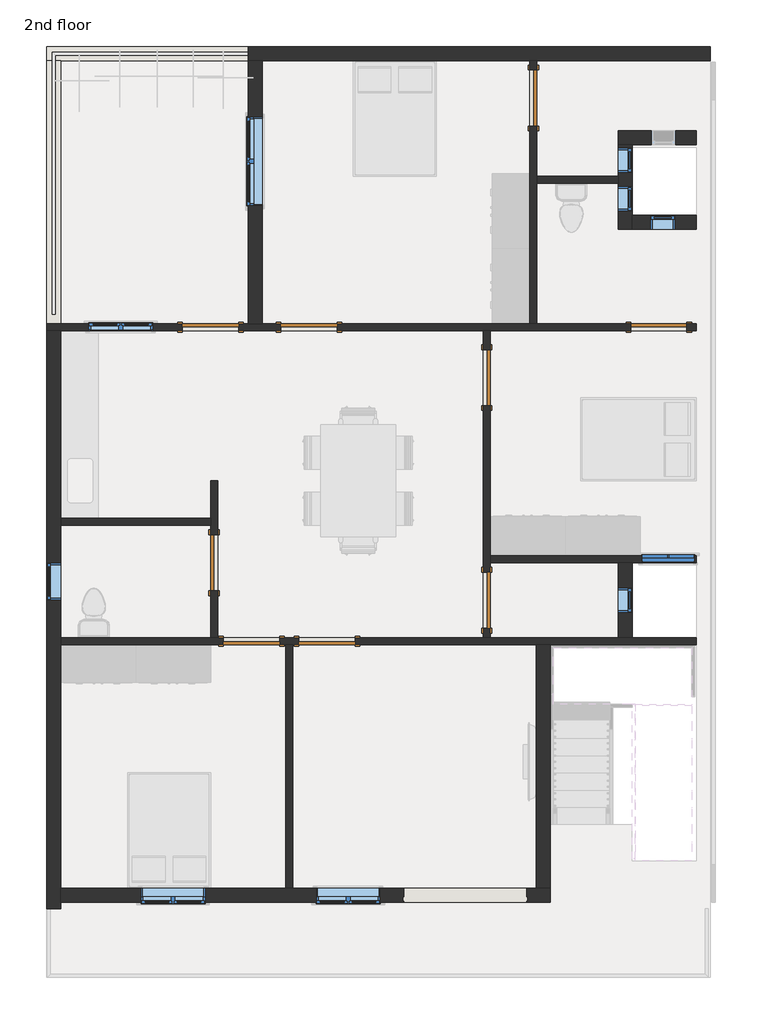
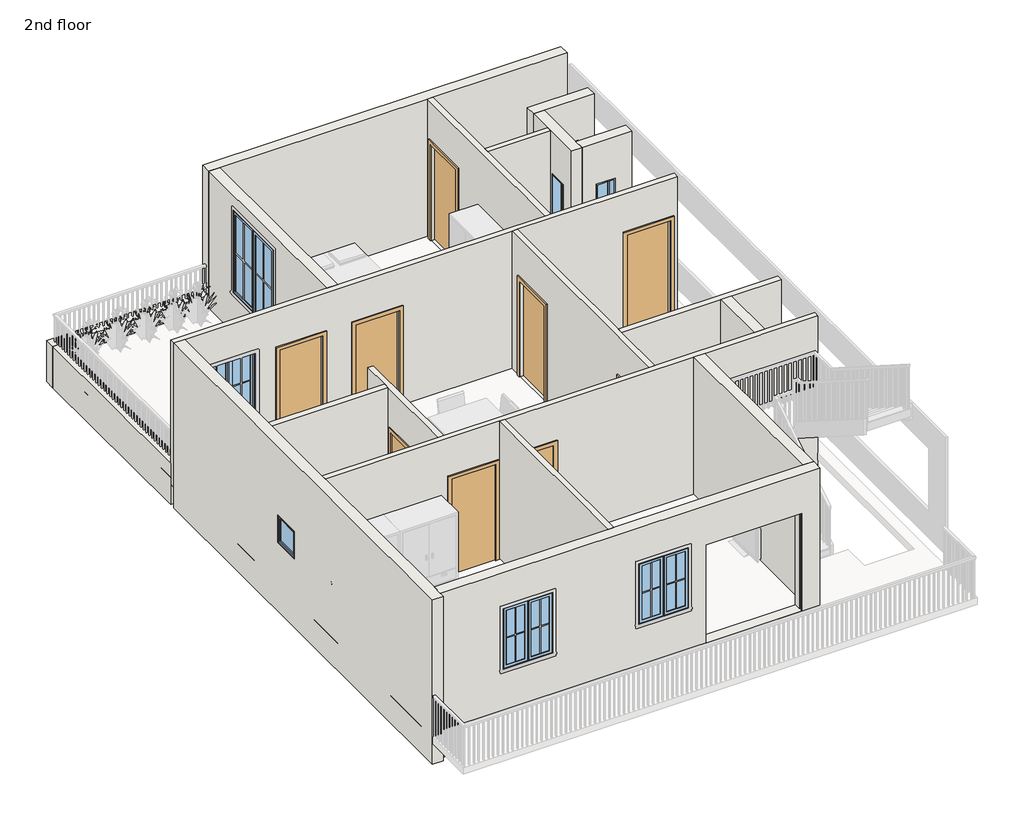
# One storey, part 1 of 5: 20 walls, 10 windows, 9 doors.
"""IFC4 building model written with IfcOpenShell, lengths in millimetres."""

from ifc_helpers import new_model, si_unit, frame, origin, place, context, project, spatial, polyline, outline, extrude, faceted_brep, transform, mapped, element, save
from components import door_305aa2a5, door_e5f9f3c4, window_aa618e30, window_cea7027f, window_80340324, window_a598f463, window_8ddb865a, window_c95ebb39, window_9ac97e1a

model = new_model("IFC4")

# Units and contexts
model_context = context("Model", 3, world=origin())
ifc_project = project(units=[si_unit("LENGTHUNIT", "METRE", prefix="MILLI")], contexts=[model_context])

# Site, building, storey
site = spatial("IfcSite", under=ifc_project)
building = spatial("IfcBuilding", under=site)
storey = spatial("IfcBuildingStorey", under=building, Name="2nd floor", Elevation=7010.4)

# Doors
placement = place(None, origin())
door_shape = door_305aa2a5(model_context)
element("IfcDoor", 1, ObjectType="Single-Flush : 36\" x 84\"", at=placement, inside=storey, context=model_context, shape_type="MappedRepresentation", body=[
    mapped(door_shape, transform((-3843.1498597, 8241.1757925, 7010.4), x_axis=(-1.0, 0.0, 0.0), y_axis=(0.0, -1.0, 0.0), z_axis=(0.0, 0.0, 1.0))),
])
element("IfcDoor", 2, ObjectType="Single-Flush : 36\" x 84\"", at=placement, inside=storey, context=model_context, shape_type="MappedRepresentation", body=[
    mapped(door_shape, transform((-953.8998597, 7422.0257925, 7010.4), x_axis=(0.0, 1.0, 0.0), y_axis=(-1.0, 0.0, 0.0), z_axis=(0.0, 0.0, 1.0))),
])
element("IfcDoor", 3, ObjectType="Single-Flush : 36\" x 84\"", at=placement, inside=storey, context=model_context, shape_type="MappedRepresentation", body=[
    mapped(door_shape, transform((-4776.5998597, 3135.7757925, 7010.4), x_axis=(1.0, 0.0, 0.0), y_axis=(0.0, 1.0, 0.0), z_axis=(0.0, 0.0, 1.0))),
])
element("IfcDoor", 4, ObjectType="Single-Flush : 36\" x 84\"", at=placement, inside=storey, context=model_context, shape_type="MappedRepresentation", body=[
    mapped(door_shape, transform((-191.8998597, 11968.6257925, 7010.4), x_axis=(0.0, 1.0, 0.0), y_axis=(-1.0, 0.0, 0.0), z_axis=(0.0, 0.0, 1.0))),
])
door_2_shape = door_e5f9f3c4(model_context)
element("IfcDoor", 5, ObjectType="Single-Flush : 36\" x 84\"", at=placement, inside=storey, context=model_context, shape_type="MappedRepresentation", body=[
    mapped(door_2_shape, transform((1846.4501403, 8241.1757925, 7010.4), x_axis=(1.0, 0.0, 0.0), y_axis=(0.0, 1.0, 0.0), z_axis=(0.0, 0.0, 1.0))),
])
element("IfcDoor", 6, ObjectType="Single-Flush : 36\" x 84\"", at=placement, inside=storey, context=model_context, shape_type="MappedRepresentation", body=[
    mapped(door_2_shape, transform((-3551.0498597, 3135.7757925, 7010.4), x_axis=(-1.0, 0.0, 0.0), y_axis=(0.0, -1.0, 0.0), z_axis=(0.0, 0.0, 1.0))),
])
element("IfcDoor", 7, ObjectType="Single-Flush : 36\" x 84\"", at=placement, inside=storey, context=model_context, shape_type="MappedRepresentation", body=[
    mapped(door_2_shape, transform((-953.8998597, 3802.5257925, 7010.4), x_axis=(0.0, -1.0, 0.0), y_axis=(1.0, 0.0, 0.0), z_axis=(0.0, 0.0, 1.0))),
])
element("IfcDoor", 8, ObjectType="Single-Flush : 36\" x 84\"", at=placement, inside=storey, context=model_context, shape_type="MappedRepresentation", body=[
    mapped(door_2_shape, transform((-5443.3498597, 8241.1757925, 7010.4), x_axis=(1.0, 0.0, 0.0), y_axis=(0.0, 1.0, 0.0), z_axis=(0.0, 0.0, 1.0))),
])
element("IfcDoor", 9, ObjectType="Single-Flush : 36\" x 84\"", at=placement, inside=storey, context=model_context, shape_type="MappedRepresentation", body=[
    mapped(door_2_shape, transform((-5386.1998597, 4412.1257925, 7010.4), x_axis=(0.0, 1.0, 0.0), y_axis=(-1.0, 0.0, 0.0), z_axis=(0.0, 0.0, 1.0))),
])

# Walls
element("IfcWall", 10, at=placement, inside=storey, context=model_context, shape_type="Brep", body=[
    faceted_brep([(-8110.3498597, 12578.2257925, 6400.8), (-7881.7498597, 12578.2257925, 6400.8), (-4833.7498597, 12578.2257925, 6400.8), (-4833.7498597, 12578.2257925, 6858.0), (-4605.1498597, 12578.2257925, 6858.0), (-4605.1498597, 12578.2257925, 7010.4), (-4719.4498597, 12578.2257925, 7010.4), (-4719.4498597, 12578.2257925, 7315.2), (-4833.7498597, 12578.2257925, 7315.2), (-7881.7498597, 12578.2257925, 7315.2), (-8110.3498597, 12578.2257925, 7315.2), (-8110.3498597, 12806.8257925, 6400.8), (-8110.3498597, 12806.8257925, 7315.2), (-4833.7498597, 12806.8257925, 7315.2), (-4719.4498597, 12806.8257925, 7315.2), (-4719.4498597, 12806.8257925, 7010.4), (-4605.1498597, 12806.8257925, 7010.4), (-4605.1498597, 12806.8257925, 6858.0), (-4833.7498597, 12806.8257925, 6858.0), (-4833.7498597, 12806.8257925, 6400.8)], [[[0, 1, 2, 3, 4, 5, 6, 7, 8, 9, 10]], [[11, 12, 13, 14, 15, 16, 17, 18, 19]], [[2, 1, 0, 11, 19]], [[10, 9, 8, 7, 14, 13, 12]], [[0, 10, 12, 11]], [[3, 2, 19, 18]], [[17, 4, 3, 18]], [[7, 6, 15, 14]], [[15, 6, 5, 16]], [[5, 4, 17, 16]]]),
])
element("IfcWall", 11, at=placement, inside=storey, context=model_context, shape_type="Brep", body=[
    faceted_brep([(-4833.7498597, 12578.2257925, 10058.4), (-4833.7498597, 12578.2257925, 7315.2), (-4833.7498597, 12578.2257925, 6858.0), (-4833.7498597, 12578.2257925, 6400.8), (-4833.7498597, 8298.3257925, 6400.8), (-4833.7498597, 8298.3257925, 10058.4), (-4833.7498597, 11663.8257925, 9753.6), (-4833.7498597, 10216.0257925, 9753.6), (-4833.7498597, 10216.0257925, 7924.8), (-4833.7498597, 11663.8257925, 7924.8), (-4605.1498597, 12578.2257925, 6400.8), (-4605.1498597, 12578.2257925, 6858.0), (-4605.1498597, 12578.2257925, 7010.4), (-4605.1498597, 12578.2257925, 10058.4), (-4605.1498597, 8298.3257925, 10058.4), (-4605.1498597, 8298.3257925, 6400.8), (-4605.1498597, 11663.8257925, 9753.6), (-4605.1498597, 11663.8257925, 7924.8), (-4605.1498597, 10216.0257925, 7924.8), (-4605.1498597, 10216.0257925, 9753.6)], [[[0, 1, 2, 3, 4, 5], [6, 7, 8, 9]], [[10, 11, 12, 13, 14, 15], [16, 17, 18, 19]], [[4, 3, 10, 15]], [[17, 16, 6, 9]], [[18, 17, 9, 8]], [[19, 18, 8, 7]], [[16, 19, 7, 6]], [[4, 15, 14, 5]], [[0, 13, 12, 11, 10, 3, 2, 1]], [[0, 5, 14, 13]]]),
])
element("IfcWall", 12, at=placement, inside=storey, context=model_context, shape_type="Brep", body=[
    faceted_brep([(2456.0501403, 8298.3257925, 6400.8), (-134.7498597, 8298.3257925, 6400.8), (-249.0498597, 8298.3257925, 6400.8), (-4605.1498597, 8298.3257925, 6400.8), (-4833.7498597, 8298.3257925, 6400.8), (-7881.7498597, 8298.3257925, 6400.8), (-7881.7498597, 8298.3257925, 6858.0), (-8110.3498597, 8298.3257925, 6858.0), (-8110.3498597, 8298.3257925, 7315.2), (-8110.3498597, 8298.3257925, 10058.4), (-4833.7498597, 8298.3257925, 10058.4), (-4605.1498597, 8298.3257925, 10058.4), (-249.0498597, 8298.3257925, 10058.4), (-134.7498597, 8298.3257925, 10058.4), (2456.0501403, 8298.3257925, 10058.4), (1389.2501403, 8298.3257925, 7010.4), (2303.6501403, 8298.3257925, 7010.4), (2303.6501403, 8298.3257925, 9144.0), (1389.2501403, 8298.3257925, 9144.0), (-3385.9498597, 8298.3257925, 7010.4), (-3385.9498597, 8298.3257925, 9144.0), (-4300.3498597, 8298.3257925, 9144.0), (-4300.3498597, 8298.3257925, 7010.4), (-5900.5498597, 8298.3257925, 7010.4), (-4986.1498597, 8298.3257925, 7010.4), (-4986.1498597, 8298.3257925, 9144.0), (-5900.5498597, 8298.3257925, 9144.0), (-6383.1498597, 8298.3257925, 9271.0), (-7424.5498597, 8298.3257925, 9271.0), (-7424.5498597, 8298.3257925, 7924.8), (-6383.1498597, 8298.3257925, 7924.8), (2456.0501403, 8184.0257925, 6400.8), (2456.0501403, 8184.0257925, 10058.4), (-896.7498597, 8184.0257925, 10058.4), (-1011.0498597, 8184.0257925, 10058.4), (-7881.7498597, 8184.0257925, 10058.4), (-8110.3498597, 8184.0257925, 10058.4), (-8110.3498597, 8184.0257925, 6858.0), (-7881.7498597, 8184.0257925, 6858.0), (-7881.7498597, 8184.0257925, 6400.8), (-1011.0498597, 8184.0257925, 6400.8), (-896.7498597, 8184.0257925, 6400.8), (1389.2501403, 8184.0257925, 7010.4), (1389.2501403, 8184.0257925, 9144.0), (2303.6501403, 8184.0257925, 9144.0), (2303.6501403, 8184.0257925, 7010.4), (-3385.9498597, 8184.0257925, 7010.4), (-4300.3498597, 8184.0257925, 7010.4), (-4300.3498597, 8184.0257925, 9144.0), (-3385.9498597, 8184.0257925, 9144.0), (-5900.5498597, 8184.0257925, 7010.4), (-5900.5498597, 8184.0257925, 9144.0), (-4986.1498597, 8184.0257925, 9144.0), (-4986.1498597, 8184.0257925, 7010.4), (-6383.1498597, 8184.0257925, 9271.0), (-6383.1498597, 8184.0257925, 7924.8), (-7424.5498597, 8184.0257925, 7924.8), (-7424.5498597, 8184.0257925, 9271.0)], [[[0, 1, 2, 3, 4, 5, 6, 7, 8, 9, 10, 11, 12, 13, 14], [15, 16, 17, 18], [19, 20, 21, 22], [23, 24, 25, 26], [27, 28, 29, 30]], [[31, 32, 33, 34, 35, 36, 37, 38, 39, 40, 41], [42, 43, 44, 45], [46, 47, 48, 49], [50, 51, 52, 53], [54, 55, 56, 57]], [[5, 4, 3, 2, 1, 0, 31, 41, 40, 39]], [[16, 15, 42, 45]], [[17, 16, 45, 44]], [[18, 17, 44, 43]], [[15, 18, 43, 42]], [[47, 46, 19, 22]], [[48, 47, 22, 21]], [[49, 48, 21, 20]], [[46, 49, 20, 19]], [[24, 23, 50, 53]], [[25, 24, 53, 52]], [[26, 25, 52, 51]], [[23, 26, 51, 50]], [[55, 54, 27, 30]], [[56, 55, 30, 29]], [[57, 56, 29, 28]], [[54, 57, 28, 27]], [[37, 7, 6, 38]], [[6, 5, 39, 38]], [[7, 37, 36, 9, 8]], [[0, 14, 32, 31]], [[14, 13, 12, 11, 10, 9, 36, 35, 34, 33, 32]]]),
])
element("IfcWall", 13, at=placement, inside=storey, context=model_context, shape_type="Brep", body=[
    faceted_brep([(2456.0501403, 11435.2257925, 6400.8), (1414.6501403, 11435.2257925, 6400.8), (1414.6501403, 11435.2257925, 6858.0), (1186.0501403, 11435.2257925, 6858.0), (1186.0501403, 11435.2257925, 10058.4), (2456.0501403, 11435.2257925, 10058.4), (1719.4501403, 11435.2257925, 9144.0), (1719.4501403, 11435.2257925, 7924.8), (2125.8501403, 11435.2257925, 7924.8), (2125.8501403, 11435.2257925, 9144.0), (2456.0501403, 11206.6257925, 6400.8), (2456.0501403, 11206.6257925, 10058.4), (1414.6501403, 11206.6257925, 10058.4), (1186.0501403, 11206.6257925, 10058.4), (1186.0501403, 11206.6257925, 6858.0), (1414.6501403, 11206.6257925, 6858.0), (1414.6501403, 11206.6257925, 6400.8), (1719.4501403, 11206.6257925, 9144.0), (2125.8501403, 11206.6257925, 9144.0), (2125.8501403, 11206.6257925, 7924.8), (1719.4501403, 11206.6257925, 7924.8)], [[[0, 1, 2, 3, 4, 5], [6, 7, 8, 9]], [[10, 11, 12, 13, 14, 15, 16], [17, 18, 19, 20]], [[1, 0, 10, 16]], [[7, 6, 17, 20]], [[8, 7, 20, 19]], [[9, 8, 19, 18]], [[6, 9, 18, 17]], [[14, 3, 2, 15]], [[2, 1, 16, 15]], [[4, 3, 14, 13]], [[0, 5, 11, 10]], [[5, 4, 13, 12, 11]]]),
])
element("IfcWall", 14, at=placement, inside=storey, context=model_context, shape_type="Brep", body=[
    faceted_brep([(1186.0501403, 11206.6257925, 6400.8), (1186.0501403, 10698.6257925, 6400.8), (1186.0501403, 10584.3257925, 6400.8), (1186.0501403, 10063.6257925, 6400.8), (1186.0501403, 10063.6257925, 6858.0), (1186.0501403, 9835.0257925, 6858.0), (1186.0501403, 9835.0257925, 10058.4), (1186.0501403, 10584.3257925, 10058.4), (1186.0501403, 10698.6257925, 10058.4), (1186.0501403, 11206.6257925, 10058.4), (1186.0501403, 11206.6257925, 6858.0), (1186.0501403, 10127.1257925, 9144.0), (1186.0501403, 10127.1257925, 7924.8), (1186.0501403, 10533.5257925, 7924.8), (1186.0501403, 10533.5257925, 9144.0), (1186.0501403, 10755.7299127, 9144.0), (1186.0501403, 10755.7299127, 7924.8), (1186.0501403, 11162.1299127, 7924.8), (1186.0501403, 11162.1299127, 9144.0), (1414.6501403, 10063.6257925, 6400.8), (1414.6501403, 11206.6257925, 6400.8), (1414.6501403, 11206.6257925, 10058.4), (1414.6501403, 10063.6257925, 10058.4), (1414.6501403, 9835.0257925, 10058.4), (1414.6501403, 9835.0257925, 6858.0), (1414.6501403, 10063.6257925, 6858.0), (1414.6501403, 10127.1257925, 7924.8), (1414.6501403, 10127.1257925, 9144.0), (1414.6501403, 10533.5257925, 9144.0), (1414.6501403, 10533.5257925, 7924.8), (1414.6501403, 10755.7299127, 7924.8), (1414.6501403, 10755.7299127, 9144.0), (1414.6501403, 11162.1299127, 9144.0), (1414.6501403, 11162.1299127, 7924.8)], [[[0, 1, 2, 3, 4, 5, 6, 7, 8, 9, 10], [11, 12, 13, 14], [15, 16, 17, 18]], [[19, 20, 21, 22, 23, 24, 25], [26, 27, 28, 29], [30, 31, 32, 33]], [[3, 2, 1, 0, 20, 19]], [[12, 11, 27, 26]], [[13, 12, 26, 29]], [[14, 13, 29, 28]], [[11, 14, 28, 27]], [[15, 31, 30, 16]], [[16, 30, 33, 17]], [[31, 15, 18, 32]], [[32, 18, 17, 33]], [[20, 0, 10, 9, 21]], [[5, 4, 25, 24]], [[4, 3, 19, 25]], [[6, 5, 24, 23]], [[21, 9, 8, 7, 6, 23, 22]]]),
])
element("IfcWall", 15, at=placement, inside=storey, context=model_context, shape_type="Brep", body=[
    faceted_brep([(1414.6501403, 9835.0257925, 10058.4), (1414.6501403, 9835.0257925, 6858.0), (1414.6501403, 9835.0257925, 6400.8), (2456.0501403, 9835.0257925, 6400.8), (2456.0501403, 9835.0257925, 10058.4), (2113.1501403, 9835.0257925, 9144.0), (2113.1501403, 9835.0257925, 7924.8), (1706.7501403, 9835.0257925, 7924.8), (1706.7501403, 9835.0257925, 9144.0), (1414.6501403, 10063.6257925, 6400.8), (1414.6501403, 10063.6257925, 10058.4), (2456.0501403, 10063.6257925, 10058.4), (2456.0501403, 10063.6257925, 6400.8), (2113.1501403, 10063.6257925, 9144.0), (1706.7501403, 10063.6257925, 9144.0), (1706.7501403, 10063.6257925, 7924.8), (2113.1501403, 10063.6257925, 7924.8)], [[[0, 1, 2, 3, 4], [5, 6, 7, 8]], [[9, 10, 11, 12], [13, 14, 15, 16]], [[3, 2, 9, 12]], [[6, 5, 13, 16]], [[7, 6, 16, 15]], [[8, 7, 15, 14]], [[5, 8, 14, 13]], [[0, 10, 9, 2, 1]], [[4, 3, 12, 11]], [[0, 4, 11, 10]]]),
])
element("IfcWall", 16, at=placement, inside=storey, context=model_context, shape_type="Brep", body=[
    faceted_brep([(-7881.7498597, 3078.6257925, 10058.4), (-7881.7498597, 3078.6257925, 6400.8), (-4224.1498597, 3078.6257925, 6400.8), (-4109.8498597, 3078.6257925, 6400.8), (-147.4498597, 3078.6257925, 6400.8), (81.1501403, 3078.6257925, 6400.8), (2456.0501403, 3078.6257925, 6400.8), (2456.0501403, 3078.6257925, 10058.4), (2430.6501403, 3078.6257925, 10058.4), (81.1501403, 3078.6257925, 10058.4), (-147.4498597, 3078.6257925, 10058.4), (-4109.8498597, 3078.6257925, 10058.4), (-4224.1498597, 3078.6257925, 10058.4), (-5233.7998597, 3078.6257925, 7010.4), (-5233.7998597, 3078.6257925, 9144.0), (-4319.3998597, 3078.6257925, 9144.0), (-4319.3998597, 3078.6257925, 7010.4), (-3093.8498597, 3078.6257925, 7010.4), (-4008.2498597, 3078.6257925, 7010.4), (-4008.2498597, 3078.6257925, 9144.0), (-3093.8498597, 3078.6257925, 9144.0), (-7881.7498597, 3192.9257925, 6400.8), (-7881.7498597, 3192.9257925, 10058.4), (-5443.3498597, 3192.9257925, 10058.4), (-5329.0498597, 3192.9257925, 10058.4), (-1011.0498597, 3192.9257925, 10058.4), (-896.7498597, 3192.9257925, 10058.4), (1186.0501403, 3192.9257925, 10058.4), (1414.6501403, 3192.9257925, 10058.4), (2456.0501403, 3192.9257925, 10058.4), (2456.0501403, 3192.9257925, 6400.8), (1414.6501403, 3192.9257925, 6400.8), (1186.0501403, 3192.9257925, 6400.8), (-896.7498597, 3192.9257925, 6400.8), (-1011.0498597, 3192.9257925, 6400.8), (-5329.0498597, 3192.9257925, 6400.8), (-5443.3498597, 3192.9257925, 6400.8), (-5233.7998597, 3192.9257925, 7010.4), (-4319.3998597, 3192.9257925, 7010.4), (-4319.3998597, 3192.9257925, 9144.0), (-5233.7998597, 3192.9257925, 9144.0), (-3093.8498597, 3192.9257925, 7010.4), (-3093.8498597, 3192.9257925, 9144.0), (-4008.2498597, 3192.9257925, 9144.0), (-4008.2498597, 3192.9257925, 7010.4)], [[[0, 1, 2, 3, 4, 5, 6, 7, 8, 9, 10, 11, 12], [13, 14, 15, 16], [17, 18, 19, 20]], [[21, 22, 23, 24, 25, 26, 27, 28, 29, 30, 31, 32, 33, 34, 35, 36], [37, 38, 39, 40], [41, 42, 43, 44]], [[6, 5, 4, 3, 2, 1, 21, 36, 35, 34, 33, 32, 31, 30]], [[38, 37, 13, 16]], [[39, 38, 16, 15]], [[40, 39, 15, 14]], [[37, 40, 14, 13]], [[18, 17, 41, 44]], [[19, 18, 44, 43]], [[20, 19, 43, 42]], [[17, 20, 42, 41]], [[0, 22, 21, 1]], [[7, 6, 30, 29]], [[0, 12, 11, 10, 9, 8, 7, 29, 28, 27, 26, 25, 24, 23, 22]]]),
])
element("IfcWall", 17, at=placement, inside=storey, context=model_context, shape_type="Brep", body=[
    faceted_brep([(-7881.7498597, -1112.3742075, 6400.8), (-147.4498597, -1112.3742075, 6400.8), (-147.4498597, -1112.3742075, 6858.0), (81.1501403, -1112.3742075, 6858.0), (81.1501403, -1112.3742075, 10058.4), (-7881.7498597, -1112.3742075, 10058.4), (-2299.8498597, -1112.3742075, 9179.9), (-299.8498597, -1112.3742075, 9179.9), (-299.8498597, -1112.3742075, 7010.4), (-2299.8498597, -1112.3742075, 7010.4), (-6573.6498597, -1112.3742075, 7924.8), (-6573.6498597, -1112.3742075, 9271.0), (-5532.2498597, -1112.3742075, 9271.0), (-5532.2498597, -1112.3742075, 7924.8), (-3725.5498597, -1112.3742075, 7924.8), (-3725.5498597, -1112.3742075, 9271.0), (-2684.1498597, -1112.3742075, 9271.0), (-2684.1498597, -1112.3742075, 7924.8), (-147.4498597, -883.7742075, 6400.8), (-4109.8498597, -883.7742075, 6400.8), (-4224.1498597, -883.7742075, 6400.8), (-7881.7498597, -883.7742075, 6400.8), (-7881.7498597, -883.7742075, 10058.4), (-4224.1498597, -883.7742075, 10058.4), (-4109.8498597, -883.7742075, 10058.4), (-147.4498597, -883.7742075, 10058.4), (81.1501403, -883.7742075, 10058.4), (81.1501403, -883.7742075, 6858.0), (-147.4498597, -883.7742075, 6858.0), (-299.8498597, -883.7742075, 9179.9), (-2299.8498597, -883.7742075, 9179.9), (-2299.8498597, -883.7742075, 7010.4), (-299.8498597, -883.7742075, 7010.4), (-6573.6498597, -883.7742075, 9271.0), (-6573.6498597, -883.7742075, 7924.8), (-5532.2498597, -883.7742075, 7924.8), (-5532.2498597, -883.7742075, 9271.0), (-3725.5498597, -883.7742075, 9271.0), (-3725.5498597, -883.7742075, 7924.8), (-2684.1498597, -883.7742075, 7924.8), (-2684.1498597, -883.7742075, 9271.0), (-2299.8498597, -1092.3742075, 9179.9), (-299.8498597, -1092.3742075, 9179.9), (-299.8498597, -1022.3742075, 9179.9), (-2299.8498597, -1022.3742075, 9179.9), (-2299.8498597, -1022.3742075, 7010.4), (-2314.8498597, -1022.3742075, 7010.4), (-2314.8498597, -1092.3742075, 7010.4), (-2299.8498597, -1092.3742075, 7010.4), (-299.8498597, -1092.3742075, 7010.4), (-284.8498597, -1092.3742075, 7010.4), (-284.8498597, -1022.3742075, 7010.4), (-299.8498597, -1022.3742075, 7010.4), (-284.8498597, -1022.3742075, 9194.9), (-2314.8498597, -1022.3742075, 9194.9), (-2314.8498597, -1092.3742075, 9194.9), (-284.8498597, -1092.3742075, 9194.9)], [[[0, 1, 2, 3, 4, 5], [6, 7, 8, 9], [10, 11, 12, 13], [14, 15, 16, 17]], [[18, 19, 20, 21, 22, 23, 24, 25, 26, 27, 28], [29, 30, 31, 32], [33, 34, 35, 36], [37, 38, 39, 40]], [[1, 0, 21, 20, 19, 18]], [[41, 42, 7, 6]], [[43, 44, 30, 29]], [[45, 46, 47, 48, 9, 8, 49, 50, 51, 52, 32, 31]], [[52, 43, 29, 32]], [[44, 45, 31, 30]], [[44, 43, 52, 51, 53, 54, 46, 45]], [[47, 46, 54, 55]], [[42, 41, 48, 47, 55, 56, 50, 49]], [[48, 41, 6, 9]], [[42, 49, 8, 7]], [[51, 50, 56, 53]], [[54, 53, 56, 55]], [[34, 33, 11, 10]], [[35, 34, 10, 13]], [[36, 35, 13, 12]], [[33, 36, 12, 11]], [[38, 37, 15, 14]], [[39, 38, 14, 17]], [[40, 39, 17, 16]], [[37, 40, 16, 15]], [[21, 0, 5, 22]], [[3, 2, 28, 27]], [[2, 1, 18, 28]], [[4, 3, 27, 26]], [[5, 4, 26, 25, 24, 23, 22]]]),
])
element("IfcWall", 18, at=placement, inside=storey, context=model_context, shape_type="SweptSolid", body=[
    extrude(outline(polyline([(-4109.8498597, 3078.6257925), (-4109.8498597, -883.7742075), (-4224.1498597, -883.7742075), (-4224.1498597, 3078.6257925), (-4109.8498597, 3078.6257925)])), frame((0.0, 0.0, 6400.8), z_axis=(0.0, 0.0, 1.0), x_axis=(1.0, 0.0, 0.0)), (0.0, 0.0, 1.0), 3657.6),
])
element("IfcWall", 19, at=placement, inside=storey, context=model_context, shape_type="Brep", body=[
    faceted_brep([(81.1501403, -883.7742075, 10058.4), (81.1501403, -883.7742075, 6858.0), (81.1501403, -883.7742075, 6400.8), (81.1501403, 3078.6257925, 6400.8), (81.1501403, 3078.6257925, 10058.4), (81.1501403, 157.6257925, 10058.4), (-147.4498597, -883.7742075, 6400.8), (-147.4498597, -883.7742075, 10058.4), (-147.4498597, 3078.6257925, 10058.4), (-147.4498597, 3078.6257925, 6400.8)], [[[0, 1, 2, 3, 4, 5]], [[6, 7, 8, 9]], [[3, 2, 6, 9]], [[3, 9, 8, 4]], [[0, 7, 6, 2, 1]], [[0, 5, 4, 8, 7]]]),
])
element("IfcWall", 20, at=placement, inside=storey, context=model_context, shape_type="SweptSolid", body=[
    extrude(outline(polyline([(3192.9257925, 6400.8), (3192.9257925, 10058.4), (4412.1257925, 10058.4), (4412.1257925, 6400.8), (3192.9257925, 6400.8)]), holes=[polyline([(3599.3257925, 8534.4), (3599.3257925, 7924.8), (4005.7257925, 7924.8), (4005.7257925, 8534.4), (3599.3257925, 8534.4)])]), frame((1186.0501403, 0.0, 0.0), z_axis=(1.0, 0.0, 0.0), x_axis=(0.0, 1.0, 0.0)), (0.0, 0.0, 1.0), 228.6),
])
element("IfcWall", 21, at=placement, inside=storey, context=model_context, shape_type="Brep", body=[
    faceted_brep([(-896.7498597, 3192.9257925, 10058.4), (-896.7498597, 3192.9257925, 6400.8), (-896.7498597, 4412.1257925, 6400.8), (-896.7498597, 4526.4257925, 6400.8), (-896.7498597, 8184.0257925, 6400.8), (-896.7498597, 8184.0257925, 10058.4), (-896.7498597, 4526.4257925, 10058.4), (-896.7498597, 4412.1257925, 10058.4), (-896.7498597, 6964.8257925, 7010.4), (-896.7498597, 6964.8257925, 9144.0), (-896.7498597, 7879.2257925, 9144.0), (-896.7498597, 7879.2257925, 7010.4), (-896.7498597, 4259.7257925, 7010.4), (-896.7498597, 3345.3257925, 7010.4), (-896.7498597, 3345.3257925, 9144.0), (-896.7498597, 4259.7257925, 9144.0), (-1011.0498597, 3192.9257925, 6400.8), (-1011.0498597, 3192.9257925, 10058.4), (-1011.0498597, 8184.0257925, 10058.4), (-1011.0498597, 8184.0257925, 6400.8), (-1011.0498597, 6964.8257925, 7010.4), (-1011.0498597, 7879.2257925, 7010.4), (-1011.0498597, 7879.2257925, 9144.0), (-1011.0498597, 6964.8257925, 9144.0), (-1011.0498597, 4259.7257925, 7010.4), (-1011.0498597, 4259.7257925, 9144.0), (-1011.0498597, 3345.3257925, 9144.0), (-1011.0498597, 3345.3257925, 7010.4)], [[[0, 1, 2, 3, 4, 5, 6, 7], [8, 9, 10, 11], [12, 13, 14, 15]], [[16, 17, 18, 19], [20, 21, 22, 23], [24, 25, 26, 27]], [[4, 3, 2, 1, 16, 19]], [[21, 20, 8, 11]], [[22, 21, 11, 10]], [[23, 22, 10, 9]], [[20, 23, 9, 8]], [[13, 12, 24, 27]], [[14, 13, 27, 26]], [[15, 14, 26, 25]], [[12, 15, 25, 24]], [[4, 19, 18, 5]], [[0, 17, 16, 1]], [[0, 7, 6, 5, 18, 17]]]),
])
element("IfcWall", 22, at=placement, inside=storey, context=model_context, shape_type="Brep", body=[
    faceted_brep([(-7881.7498597, -1213.9742075, 6400.8), (-7881.7498597, -1112.3742075, 6400.8), (-7881.7498597, -883.7742075, 6400.8), (-7881.7498597, 3078.6257925, 6400.8), (-7881.7498597, 3192.9257925, 6400.8), (-7881.7498597, 5021.7257925, 6400.8), (-7881.7498597, 5136.0257925, 6400.8), (-7881.7498597, 8184.0257925, 6400.8), (-7881.7498597, 8184.0257925, 10058.4), (-7881.7498597, 5136.0257925, 10058.4), (-7881.7498597, 5021.7257925, 10058.4), (-7881.7498597, 3192.9257925, 10058.4), (-7881.7498597, 3078.6257925, 10058.4), (-7881.7498597, -883.7742075, 10058.4), (-7881.7498597, -1112.3742075, 10058.4), (-7881.7498597, -1213.9742075, 10058.4), (-7881.7498597, 4412.1257925, 8534.4), (-7881.7498597, 4412.1257925, 7924.8), (-7881.7498597, 3802.5257925, 7924.8), (-7881.7498597, 3802.5257925, 8534.4), (-8110.3498597, -1213.9742075, 6400.8), (-8110.3498597, -1213.9742075, 10058.4), (-8110.3498597, 8184.0257925, 10058.4), (-8110.3498597, 8184.0257925, 6858.0), (-8110.3498597, 8184.0257925, 6400.8), (-8110.3498597, 4412.1257925, 8534.4), (-8110.3498597, 3802.5257925, 8534.4), (-8110.3498597, 3802.5257925, 7924.8), (-8110.3498597, 4412.1257925, 7924.8)], [[[0, 1, 2, 3, 4, 5, 6, 7, 8, 9, 10, 11, 12, 13, 14, 15], [16, 17, 18, 19]], [[20, 21, 22, 23, 24], [25, 26, 27, 28]], [[7, 6, 5, 4, 3, 2, 1, 0, 20, 24]], [[0, 15, 21, 20]], [[16, 19, 26, 25]], [[19, 18, 27, 26]], [[18, 17, 28, 27]], [[17, 16, 25, 28]], [[7, 24, 23, 22, 8]], [[15, 14, 13, 12, 11, 10, 9, 8, 22, 21]]]),
])
element("IfcWall", 23, at=placement, inside=storey, context=model_context, shape_type="Brep", body=[
    faceted_brep([(-7881.7498597, 8298.3257925, 7315.2), (-7881.7498597, 8298.3257925, 6400.8), (-7881.7498597, 12578.2257925, 6400.8), (-7881.7498597, 12578.2257925, 7315.2), (-8110.3498597, 8298.3257925, 6400.8), (-8110.3498597, 8298.3257925, 6858.0), (-8110.3498597, 8298.3257925, 7315.2), (-8110.3498597, 12578.2257925, 7315.2), (-8110.3498597, 12578.2257925, 6400.8)], [[[0, 1, 2, 3]], [[4, 5, 6, 7, 8]], [[2, 1, 4, 8]], [[0, 3, 7, 6]], [[3, 2, 8, 7]], [[0, 6, 5, 4, 1]]]),
])
element("IfcWall", 24, at=placement, inside=storey, context=model_context, shape_type="Brep", body=[
    faceted_brep([(-4719.4498597, 12578.2257925, 7010.4), (-4605.1498597, 12578.2257925, 7010.4), (2684.6501403, 12578.2257925, 7010.4), (2684.6501403, 12578.2257925, 10058.4), (-134.7498597, 12578.2257925, 10058.4), (-249.0498597, 12578.2257925, 10058.4), (-4605.1498597, 12578.2257925, 10058.4), (-4833.7498597, 12578.2257925, 10058.4), (-4833.7498597, 12578.2257925, 7315.2), (-4719.4498597, 12578.2257925, 7315.2), (-4719.4498597, 12806.8257925, 7010.4), (-4719.4498597, 12806.8257925, 7315.2), (-4833.7498597, 12806.8257925, 7315.2), (-4833.7498597, 12806.8257925, 10058.4), (2684.6501403, 12806.8257925, 10058.4), (2684.6501403, 12806.8257925, 7010.4), (-4605.1498597, 12806.8257925, 7010.4)], [[[0, 1, 2, 3, 4, 5, 6, 7, 8, 9]], [[10, 11, 12, 13, 14, 15, 16]], [[2, 1, 0, 10, 16, 15]], [[0, 9, 11, 10]], [[8, 12, 11, 9]], [[3, 2, 15, 14]], [[8, 7, 13, 12]], [[7, 6, 5, 4, 3, 14, 13]]]),
])
element("IfcWall", 25, at=placement, inside=storey, context=model_context, shape_type="Brep", body=[
    faceted_brep([(-249.0498597, 12578.2257925, 10058.4), (-249.0498597, 12578.2257925, 6400.8), (-249.0498597, 8298.3257925, 6400.8), (-249.0498597, 8298.3257925, 10058.4), (-249.0498597, 11511.4257925, 7010.4), (-249.0498597, 12425.8257925, 7010.4), (-249.0498597, 12425.8257925, 9144.0), (-249.0498597, 11511.4257925, 9144.0), (-134.7498597, 12578.2257925, 6400.8), (-134.7498597, 12578.2257925, 10058.4), (-134.7498597, 10698.6257925, 10058.4), (-134.7498597, 10584.3257925, 10058.4), (-134.7498597, 8298.3257925, 10058.4), (-134.7498597, 8298.3257925, 6400.8), (-134.7498597, 10584.3257925, 6400.8), (-134.7498597, 10698.6257925, 6400.8), (-134.7498597, 11511.4257925, 7010.4), (-134.7498597, 11511.4257925, 9144.0), (-134.7498597, 12425.8257925, 9144.0), (-134.7498597, 12425.8257925, 7010.4)], [[[0, 1, 2, 3], [4, 5, 6, 7]], [[8, 9, 10, 11, 12, 13, 14, 15], [16, 17, 18, 19]], [[2, 1, 8, 15, 14, 13]], [[5, 4, 16, 19]], [[6, 5, 19, 18]], [[7, 6, 18, 17]], [[4, 7, 17, 16]], [[0, 3, 12, 11, 10, 9]], [[2, 13, 12, 3]], [[0, 9, 8, 1]]]),
])
element("IfcWall", 26, at=placement, inside=storey, context=model_context, shape_type="SweptSolid", body=[
    extrude(outline(polyline([(-134.7498597, 10698.6257925), (1186.0501403, 10698.6257925), (1186.0501403, 10584.3257925), (-134.7498597, 10584.3257925), (-134.7498597, 10698.6257925)])), frame((0.0, 0.0, 6400.8), z_axis=(0.0, 0.0, 1.0), x_axis=(1.0, 0.0, 0.0)), (0.0, 0.0, 1.0), 3657.6),
])
element("IfcWall", 27, at=placement, inside=storey, context=model_context, shape_type="Brep", body=[
    faceted_brep([(2456.0501403, 4526.4257925, 6400.8), (-896.7498597, 4526.4257925, 6400.8), (-896.7498597, 4526.4257925, 10058.4), (2456.0501403, 4526.4257925, 10058.4), (2430.6501403, 4526.4257925, 8229.6), (1567.0501403, 4526.4257925, 8229.6), (1567.0501403, 4526.4257925, 7315.2), (2430.6501403, 4526.4257925, 7315.2), (2456.0501403, 4412.1257925, 6400.8), (2456.0501403, 4412.1257925, 10058.4), (1414.6501403, 4412.1257925, 10058.4), (1186.0501403, 4412.1257925, 10058.4), (-896.7498597, 4412.1257925, 10058.4), (-896.7498597, 4412.1257925, 6400.8), (1186.0501403, 4412.1257925, 6400.8), (1414.6501403, 4412.1257925, 6400.8), (2430.6501403, 4412.1257925, 8229.6), (2430.6501403, 4412.1257925, 7315.2), (1567.0501403, 4412.1257925, 7315.2), (1567.0501403, 4412.1257925, 8229.6)], [[[0, 1, 2, 3], [4, 5, 6, 7]], [[8, 9, 10, 11, 12, 13, 14, 15], [16, 17, 18, 19]], [[1, 0, 8, 15, 14, 13]], [[17, 16, 4, 7]], [[18, 17, 7, 6]], [[19, 18, 6, 5]], [[16, 19, 5, 4]], [[3, 2, 12, 11, 10, 9]], [[1, 13, 12, 2]], [[0, 3, 9, 8]]]),
])
element("IfcWall", 28, at=placement, inside=storey, context=model_context, shape_type="SweptSolid", body=[
    extrude(outline(polyline([(-5443.3498597, 5021.7257925), (-7881.7498597, 5021.7257925), (-7881.7498597, 5136.0257925), (-5443.3498597, 5136.0257925), (-5443.3498597, 5021.7257925)])), frame((0.0, 0.0, 6400.8), z_axis=(0.0, 0.0, 1.0), x_axis=(1.0, 0.0, 0.0)), (0.0, 0.0, 1.0), 3657.6),
])
element("IfcWall", 29, at=placement, inside=storey, context=model_context, shape_type="Brep", body=[
    faceted_brep([(-5329.0498597, 3192.9257925, 10058.4), (-5329.0498597, 3192.9257925, 6400.8), (-5329.0498597, 5745.6257925, 6400.8), (-5329.0498597, 5745.6257925, 10058.4), (-5329.0498597, 3954.9257925, 7010.4), (-5329.0498597, 3954.9257925, 9144.0), (-5329.0498597, 4869.3257925, 9144.0), (-5329.0498597, 4869.3257925, 7010.4), (-5443.3498597, 3192.9257925, 6400.8), (-5443.3498597, 3192.9257925, 10058.4), (-5443.3498597, 5021.7257925, 10058.4), (-5443.3498597, 5136.0257925, 10058.4), (-5443.3498597, 5745.6257925, 10058.4), (-5443.3498597, 5745.6257925, 6400.8), (-5443.3498597, 5136.0257925, 6400.8), (-5443.3498597, 5021.7257925, 6400.8), (-5443.3498597, 3954.9257925, 7010.4), (-5443.3498597, 4869.3257925, 7010.4), (-5443.3498597, 4869.3257925, 9144.0), (-5443.3498597, 3954.9257925, 9144.0)], [[[0, 1, 2, 3], [4, 5, 6, 7]], [[8, 9, 10, 11, 12, 13, 14, 15], [16, 17, 18, 19]], [[2, 1, 8, 15, 14, 13]], [[3, 2, 13, 12]], [[17, 16, 4, 7]], [[18, 17, 7, 6]], [[19, 18, 6, 5]], [[16, 19, 5, 4]], [[0, 3, 12, 11, 10, 9]], [[0, 9, 8, 1]]]),
])

# Windows
window_shape = window_aa618e30(model_context)
element("IfcWindow", 30, ObjectType="Fixed : 16\" x 24\"", at=placement, inside=storey, context=model_context, shape_type="MappedRepresentation", body=[
    mapped(window_shape, transform((1300.3501403, 3764.4257925, 7010.4), x_axis=(0.0, -1.0, 0.0), y_axis=(1.0, 0.0, 0.0), z_axis=(0.0, 0.0, 1.0))),
])
window_2_shape = window_cea7027f(model_context)
element("IfcWindow", 31, ObjectType="Fixed : 16\" x 48\"", at=placement, inside=storey, context=model_context, shape_type="MappedRepresentation", body=[
    mapped(window_2_shape, transform((1948.0501403, 9949.3257925, 7010.4), x_axis=(1.0, 0.0, 0.0), y_axis=(0.0, 1.0, 0.0), z_axis=(0.0, 0.0, 1.0))),
])
element("IfcWindow", 32, ObjectType="Fixed : 16\" x 48\"", at=placement, inside=storey, context=model_context, shape_type="MappedRepresentation", body=[
    mapped(window_2_shape, transform((1300.3501403, 10292.2257925, 7010.4), x_axis=(0.0, -1.0, 0.0), y_axis=(1.0, 0.0, 0.0), z_axis=(0.0, 0.0, 1.0))),
])
element("IfcWindow", 33, ObjectType="Fixed : 16\" x 48\"", at=placement, inside=storey, context=model_context, shape_type="MappedRepresentation", body=[
    mapped(window_2_shape, transform((1300.3501403, 10920.8299127, 7010.4), x_axis=(0.0, -1.0, 0.0), y_axis=(1.0, 0.0, 0.0), z_axis=(0.0, 0.0, 1.0))),
])
window_3_shape = window_80340324(model_context)
element("IfcWindow", 34, ObjectType="Fixed : 24\" x 24\"", at=placement, inside=storey, context=model_context, shape_type="MappedRepresentation", body=[
    mapped(window_3_shape, transform((-7996.0498597, 4145.4257925, 7010.4), x_axis=(0.0, 1.0, 0.0), y_axis=(-1.0, 0.0, 0.0), z_axis=(0.0, 0.0, 1.0))),
])
window_4_shape = window_a598f463(model_context)
element("IfcWindow", 35, ObjectType="Window-Casement-Double : 34\" x 36\"", at=placement, inside=storey, context=model_context, shape_type="MappedRepresentation", body=[
    mapped(window_4_shape, transform((1998.8501403, 4469.2757925, 6400.8), x_axis=(1.0, 0.0, 0.0), y_axis=(0.0, 1.0, 0.0), z_axis=(0.0, 0.0, 1.0))),
])
window_5_shape = window_8ddb865a(model_context)
element("IfcWindow", 36, ObjectType="Window-Casement-Double : 41\" x 53\"", at=placement, inside=storey, context=model_context, shape_type="MappedRepresentation", body=[
    mapped(window_5_shape, transform((-6903.8498597, 8241.1757925, 7010.4), x_axis=(1.0, 0.0, 0.0), y_axis=(0.0, 1.0, 0.0), z_axis=(0.0, 0.0, 1.0))),
])
window_6_shape = window_c95ebb39(model_context)
element("IfcWindow", 37, ObjectType="Window-Casement-Double : 41\" x 53\"", at=placement, inside=storey, context=model_context, shape_type="MappedRepresentation", body=[
    mapped(window_6_shape, transform((-6052.9498597, -998.0742075, 7010.4), x_axis=(-1.0, 0.0, 0.0), y_axis=(0.0, -1.0, 0.0), z_axis=(0.0, 0.0, 1.0))),
])
element("IfcWindow", 38, ObjectType="Window-Casement-Double : 41\" x 53\"", at=placement, inside=storey, context=model_context, shape_type="MappedRepresentation", body=[
    mapped(window_6_shape, transform((-3204.8498597, -998.0742075, 7010.4), x_axis=(-1.0, 0.0, 0.0), y_axis=(0.0, -1.0, 0.0), z_axis=(0.0, 0.0, 1.0))),
])
window_7_shape = window_9ac97e1a(model_context)
element("IfcWindow", 39, ObjectType="Window-Casement-Double : 57\" x 72\"", at=placement, inside=storey, context=model_context, shape_type="MappedRepresentation", body=[
    mapped(window_7_shape, transform((-4719.4498597, 10939.9257925, 7010.4), x_axis=(0.0, 1.0, 0.0), y_axis=(-1.0, 0.0, 0.0), z_axis=(0.0, 0.0, 1.0))),
])

save(model, "model.ifc")

# Revit data of these elements
# Type "Single-Flush : 36\" x 84\""
#   Type Mark = "1"
#   Construction Type Id = "MDOOR"
#   Assembly Code = "C1020"
#   Analytic Construction = "Metal"
#   Thickness = 0' - 2"
#   Heat Transfer Coefficient (U) = 0.651978 BTU/(h·ft²·°F)
#   Height = 7' - 0"
#   Trim Projection Ext = 0' - 1"
#   Trim Projection Int = 0' - 1"
#   Trim Width = 0' - 3"
#   Width = 3' - 0"
#   Define Thermal Properties by = 1
#   Define Thermal Properties by = 1
#   Door Material = Door - Panel
#   Frame Material = Door - Frame
#   Visual Light Transmittance = 0
#   Solar Heat Gain Coefficient = 0
#   Function = (empty or 0)
#   Wall Closure = (empty or 0)
# Type
#   Assembly Code = "B2010"
#   Layers, outside or top first: 0' - 9" no material (function 1)
# Type
#   Assembly Code = "B2010"
#   Layers, outside or top first: 0' - 4 1/2" no material (function 1)
# Type "Fixed : 16\" x 24\""
#   Type Mark = "4"
#   Construction Type Id = "GSP4R"
#   Assembly Code = "B2020100"
#   Analytic Construction = "1/8 in Pilkington single glazing"
#   Visual Light Transmittance = 0.9
#   Solar Heat Gain Coefficient = 0.78
#   Heat Transfer Coefficient (U) = 0.6496 BTU/(h·ft²·°F)
#   Height = 2' - 0"
#   Default Sill Height = 3' - 0"
#   Width = 1' - 4"
#   Window Inset = 0' - 0 3/4"
#   Define Thermal Properties by = 1
#   Define Thermal Properties by = 1
#   Glass Pane Material = Glass
#   Sash Material = Sash
#   Wall Closure = (empty or 0)
# Type "Fixed : 16\" x 48\""
#   Type Mark = "5"
#   Construction Type Id = "GSP4R"
#   Assembly Code = "B2020100"
#   Analytic Construction = "1/8 in Pilkington single glazing"
#   Visual Light Transmittance = 0.9
#   Solar Heat Gain Coefficient = 0.78
#   Heat Transfer Coefficient (U) = 0.6496 BTU/(h·ft²·°F)
#   Height = 4' - 0"
#   Default Sill Height = 3' - 0"
#   Width = 1' - 4"
#   Window Inset = 0' - 0 3/4"
#   Define Thermal Properties by = 1
#   Define Thermal Properties by = 1
#   Glass Pane Material = Glass
#   Sash Material = Sash
#   Wall Closure = (empty or 0)
# Type "Fixed : 24\" x 24\""
#   Type Mark = "3"
#   Construction Type Id = "GSP4R"
#   Assembly Code = "B2020100"
#   Analytic Construction = "1/8 in Pilkington single glazing"
#   Visual Light Transmittance = 0.9
#   Solar Heat Gain Coefficient = 0.78
#   Heat Transfer Coefficient (U) = 0.6496 BTU/(h·ft²·°F)
#   Height = 2' - 0"
#   Default Sill Height = 3' - 0"
#   Width = 2' - 0"
#   Window Inset = 0' - 0 3/4"
#   Define Thermal Properties by = 1
#   Define Thermal Properties by = 1
#   Glass Pane Material = Glass
#   Sash Material = Sash
#   Wall Closure = (empty or 0)
# Type "Window-Casement-Double : 34\" x 36\""
#   Type Mark = "14"
#   Fire Rating = "0.5h"
#   Assembly Code = "B2020100"
#   Analytic Construction = "Double glazing - domestic"
#   Frame Extension [instance default] = 0' - 0 1/4"
#   Window Inset [instance default] = 0' - 0"
#   Wall Thickness [instance default] = 0' - 6"
#   Interior Wall Closure [instance default] = 0' - 2 1/4"
#   Half Width = 1' - 5"
#   Visual Light Transmittance = 0.81
#   Thermal Resistance (R) = 1.8146 (h·ft²·°F)/BTU
#   Solar Heat Gain Coefficient = 0.76
#   Rough Width = 2' - 10 1/2"
#   Rough Height = 3' - 0 1/2"
#   Height = 3' - 0"
#   Heat Transfer Coefficient (U) = 0.5511 BTU/(h·ft²·°F)
#   Exterior Wall Closure [instance default] = 0' - 1 1/4"
#   Extension Jamb [instance default] = 0' - 2 1/4"
#   Default Sill Height = 3' - 0"
#   Width = 2' - 10"
#   Define Thermal Properties by = 0
#   Muntin Visibility = yes
#   Interior Trim Visibility [instance default] = yes
#   Exterior Trim Visibility [instance default] = yes
#   Extension Jamb Visibility [instance default] = yes
#   Interior Trim Material = Wood - Stained
#   Muntin Pattern = Muntin Pattern_2x2 : Muntin Pattern_2x2
#   Interior Trim = Trim-Window-Interior-Flat : Picture Frame
#   Interior Frame Material = Wood - Stained
#   Glass Panel Material = Glass
#   Exterior Trim Material = Clad - White
#   Exterior Trim = Trim-Window-Exterior-Flat : with Sill
#   Exterior Frame Material = Clad - White
#   Wall Closure = (empty or 0)
# Type "Window-Casement-Double : 41\" x 53\""
#   Type Mark = "15"
#   Fire Rating = "0.5h"
#   Assembly Code = "B2020100"
#   Analytic Construction = "Double glazing - domestic"
#   Frame Extension [instance default] = 0' - 0 1/4"
#   Window Inset [instance default] = 0' - 0"
#   Wall Thickness [instance default] = 0' - 6"
#   Interior Wall Closure [instance default] = 0' - 2 1/4"
#   Half Width = 1' - 8 1/2"
#   Visual Light Transmittance = 0.81
#   Thermal Resistance (R) = 1.8146 (h·ft²·°F)/BTU
#   Solar Heat Gain Coefficient = 0.76
#   Rough Width = 3' - 5 1/2"
#   Rough Height = 4' - 5 1/2"
#   Height = 4' - 5"
#   Heat Transfer Coefficient (U) = 0.5511 BTU/(h·ft²·°F)
#   Exterior Wall Closure [instance default] = 0' - 1 1/4"
#   Extension Jamb [instance default] = 0' - 2 1/4"
#   Default Sill Height = 3' - 0"
#   Width = 3' - 5"
#   Define Thermal Properties by = 0
#   Muntin Visibility = yes
#   Interior Trim Visibility [instance default] = yes
#   Exterior Trim Visibility [instance default] = yes
#   Extension Jamb Visibility [instance default] = yes
#   Interior Trim Material = Wood - Stained
#   Muntin Pattern = Muntin Pattern_2x2 : Muntin Pattern_2x2
#   Interior Trim = Trim-Window-Interior-Flat : Picture Frame
#   Interior Frame Material = Wood - Stained
#   Glass Panel Material = Glass
#   Exterior Trim Material = Clad - White
#   Exterior Trim = Trim-Window-Exterior-Flat : with Sill
#   Exterior Frame Material = Clad - White
#   Wall Closure = (empty or 0)
# Type "Window-Casement-Double : 57\" x 72\""
#   Type Mark = "17"
#   Fire Rating = "0.5h"
#   Assembly Code = "B2020100"
#   Analytic Construction = "Double glazing - domestic"
#   Frame Extension [instance default] = 0' - 0 1/4"
#   Window Inset [instance default] = 0' - 0"
#   Wall Thickness [instance default] = 0' - 6"
#   Interior Wall Closure [instance default] = 0' - 2 1/4"
#   Half Width = 2' - 4 1/2"
#   Visual Light Transmittance = 0.81
#   Thermal Resistance (R) = 1.8146 (h·ft²·°F)/BTU
#   Solar Heat Gain Coefficient = 0.76
#   Rough Width = 4' - 9 1/2"
#   Rough Height = 6' - 0 1/2"
#   Height = 6' - 0"
#   Heat Transfer Coefficient (U) = 0.5511 BTU/(h·ft²·°F)
#   Exterior Wall Closure [instance default] = 0' - 1 1/4"
#   Extension Jamb [instance default] = 0' - 2 1/4"
#   Default Sill Height = 3' - 0"
#   Width = 4' - 9"
#   Define Thermal Properties by = 0
#   Muntin Visibility = yes
#   Interior Trim Visibility [instance default] = yes
#   Exterior Trim Visibility [instance default] = yes
#   Extension Jamb Visibility [instance default] = yes
#   Interior Trim Material = Wood - Stained
#   Muntin Pattern = Muntin Pattern_2x2 : Muntin Pattern_2x2
#   Interior Trim = Trim-Window-Interior-Flat : Picture Frame
#   Interior Frame Material = Wood - Stained
#   Glass Panel Material = Glass
#   Exterior Trim Material = Clad - White
#   Exterior Trim = Trim-Window-Exterior-Flat : with Sill
#   Exterior Frame Material = Clad - White
#   Wall Closure = (empty or 0)
# Elements 1, 2, 3, 4, 5, 6, 7, 8, 9 (IfcDoor, "Single-Flush : 36\" x 84\"")
#   Phase Created = New Construction
#   Materials on its faces: "Door - Frame", "Door - Panel"
# Elements 10, 23 (IfcWall)
#   built-in parameter 1001111 = -2' - 0"
#   Top Offset = 0' - 0"
#   Base Offset = -2' - 0"
#   Unconnected Height = 3' - 0"
#   wall height = 3' - 0"
#   Phase Created = New Construction
#   Base Constraint = 2nd floor
#   Materials on its faces: "Default Wall"
# Elements 11, 12, 13, 14, 15, 16, 17, 18, 19, 20, 21, 22, 25, 26, 27, 28, 29 (IfcWall)
#   built-in parameter 1001111 = -2' - 0"
#   Top Offset = 0' - 0"
#   Base Offset = -2' - 0"
#   wall height = 12' - 0"
#   Phase Created = New Construction
#   Base Constraint = 2nd floor
#   Top Constraint = terrace
#   Materials on its faces: "Default Wall"
# Element 24 (IfcWall)
#   Top Offset = 0' - 0"
#   Base Offset = 0' - 0"
#   wall height = 10' - 0"
#   Phase Created = New Construction
#   Base Constraint = 2nd floor
#   Top Constraint = terrace
#   Materials on its faces: "Default Wall"
# Element 30 (IfcWindow, "Fixed : 16\" x 24\"")
#   Mark = "31"
#   Phase Created = New Construction
#   Materials on its faces: "Sash", "Glass"
# Element 31 (IfcWindow, "Fixed : 16\" x 48\"")
#   Mark = "29"
#   Phase Created = New Construction
#   Materials on its faces: "Sash", "Glass"
# Element 32 (IfcWindow, "Fixed : 16\" x 48\"")
#   Mark = "33"
#   Phase Created = New Construction
#   Materials on its faces: "Sash", "Glass"
# Element 33 (IfcWindow, "Fixed : 16\" x 48\"")
#   Mark = "34"
#   Phase Created = New Construction
#   Materials on its faces: "Sash", "Glass"
# Element 34 (IfcWindow, "Fixed : 24\" x 24\"")
#   Mark = "32"
#   Phase Created = New Construction
#   Materials on its faces: "Sash", "Glass"
# Element 35 (IfcWindow, "Window-Casement-Double : 34\" x 36\"")
#   Mark = "41"
#   Window Inset = 0' - 0"
#   Interior Wall Closure = 0' - 2 1/4"
#   Frame Extension = 0' - 0 1/4"
#   Exterior Wall Closure = 0' - 1 1/4"
#   Interior Trim Visibility = yes
#   Exterior Trim Visibility = yes
#   Phase Created = New Construction
#   Materials on its faces: "Wood - Stained", "Glass", "Clad - White"
# Element 36 (IfcWindow, "Window-Casement-Double : 41\" x 53\"")
#   Mark = "26"
#   Window Inset = 0' - 0"
#   Interior Wall Closure = 0' - 2 1/4"
#   Frame Extension = 0' - 0 1/4"
#   Exterior Wall Closure = 0' - 1 1/4"
#   Interior Trim Visibility = yes
#   Exterior Trim Visibility = yes
#   Phase Created = New Construction
#   Materials on its faces: "Wood - Stained", "Glass", "Clad - White"
# Element 37 (IfcWindow, "Window-Casement-Double : 41\" x 53\"")
#   Mark = "27"
#   Window Inset = 0' - 0"
#   Interior Wall Closure = 0' - 2 1/4"
#   Frame Extension = 0' - 0 1/4"
#   Exterior Wall Closure = 0' - 1 1/4"
#   Interior Trim Visibility = yes
#   Exterior Trim Visibility = yes
#   Phase Created = New Construction
#   Materials on its faces: "Wood - Stained", "Glass", "Clad - White"
# Element 38 (IfcWindow, "Window-Casement-Double : 41\" x 53\"")
#   Mark = "28"
#   Window Inset = 0' - 0"
#   Interior Wall Closure = 0' - 2 1/4"
#   Frame Extension = 0' - 0 1/4"
#   Exterior Wall Closure = 0' - 1 1/4"
#   Interior Trim Visibility = yes
#   Exterior Trim Visibility = yes
#   Phase Created = New Construction
#   Materials on its faces: "Wood - Stained", "Glass", "Clad - White"
# Element 39 (IfcWindow, "Window-Casement-Double : 57\" x 72\"")
#   Mark = "25"
#   Window Inset = 0' - 0"
#   Interior Wall Closure = 0' - 2 1/4"
#   Frame Extension = 0' - 0 1/4"
#   Exterior Wall Closure = 0' - 1 1/4"
#   Interior Trim Visibility = yes
#   Exterior Trim Visibility = yes
#   Phase Created = New Construction
#   Materials on its faces: "Wood - Stained", "Glass", "Clad - White"
# Materials
#   "Door - Panel": class "Wood", colour RGB 210 159 95, transparency 0, Cost = 0
#   "Door - Frame": colour RGB 118 70 51, transparency 0, Cost = 0
#   "Glass": class "Glass", colour RGB 0 128 192, transparency 0.75, Description = "Soda Lime Glass", Cost = 0
#   "Sash": class "Wood", colour RGB 224 178 126, transparency 0, Cost = 0
#   "Wood - Stained": class "Wood", colour RGB 224 178 126, transparency 0, Cost = 0
#   "Clad - White": class "Wood", colour RGB 242 242 238, transparency 0, Cost = 0
#   "Default Wall": colour RGB 128 128 128, transparency 0, Cost = 0
# Area at (-2874.136, 8895.545) mm, upper offset 0' - 0", lower offset 0' - 0"
#   Number = "2"
#   Name = "Area"
# Area at (-6526.157, 10337.132) mm, upper offset 0' - 0", lower offset 0' - 0"
#   Number = "3"
#   Name = "Area"
# Area at (-2201.395, 1207.079) mm, upper offset 0' - 0", lower offset 0' - 0"
#   Number = "4"
#   Name = "Area"
# Room at (-6359.578, 10995.061) mm, phase "New Construction", upper level "2nd floor", upper offset 8' - 0", lower offset 0' - 0"
#   Number = "1"
#   Name = "Room"
# Room at (-3073.639, 9735.869) mm, phase "New Construction", upper level "2nd floor", upper offset 8' - 0", lower offset 0' - 0"
#   Number = "2"
#   Name = "Room"
# Room at (-5538.093, 6224.13) mm, phase "New Construction", upper level "2nd floor", upper offset 8' - 0", lower offset 0' - 0"
#   Number = "3"
#   Name = "Room"
# Room at (-5980.431, 1769.154) mm, phase "New Construction", upper level "2nd floor", upper offset 8' - 0", lower offset 0' - 0"
#   Number = "4"
#   Name = "Room"
# Room at (-1620.242, 2179.897) mm, phase "New Construction", upper level "2nd floor", upper offset 8' - 0", lower offset 0' - 0"
#   Number = "5"
#   Name = "Room"
# Room at (686.234, 7483.321) mm, phase "New Construction", upper level "2nd floor", upper offset 8' - 0", lower offset 0' - 0"
#   Number = "6"
#   Name = "Room"
# Room at (686.234, 9735.869) mm, phase "New Construction", upper level "2nd floor", upper offset 8' - 0", lower offset 0' - 0"
#   Number = "7"
#   Name = "Room"
# Room at (1065.381, 11468.994) mm, phase "New Construction", upper level "2nd floor", upper offset 8' - 0", lower offset 0' - 0"
#   Number = "8"
#   Name = "Room"
